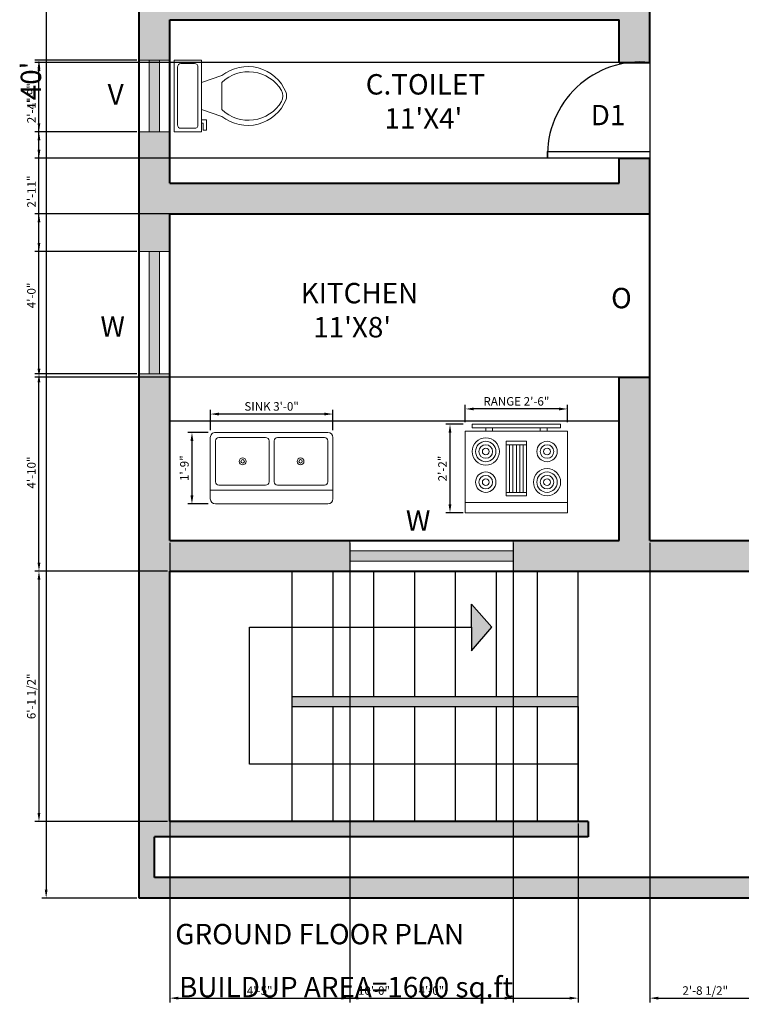
# Model space of a CAD drawing. Units: inches. Extents: x 4432 to 4859, y 8121 to 8698.
# Tile 1 of 4: x 4432 to 4644, y 8121 to 8410. Entities that reach past the tile are written whole.
import ezdxf

# ---------------------------------------------------------------- set-up
doc = ezdxf.new("R2010")
doc.units = ezdxf.units.IN
for name, color, linetype, lineweight in [('A-ANNO-DIMS', 2, 'Continuous', 18), ('A-ANNO-TEXT', 7, 'Continuous', 18), ('A-AREA-IDEN', 4, 'Continuous', 18), ('A-DOOR', 3, 'Continuous', 25), ('A-EQPM', 8, 'Continuous', 18), ('A-FLOR-CASE', 8, 'Continuous', 25), ('A-FLOR-FIXT', 9, 'Continuous', 18), ('A-FLOR-STRS', 7, 'Continuous', 25), ('A-FURN-PATT', 8, 'Continuous', 13), ('A-GLAZ', 4, 'Continuous', 20), ('A-GLAZ-PATT', 4, 'Continuous', 13), ('A-WALL', 7, 'Continuous', 40)]:
    doc.layers.add(name, color=color, linetype=linetype, lineweight=lineweight)
doc.layers.add('A-FLOR-PATT', color=219, linetype='Continuous', lineweight=13, true_color=0x642165)
doc.layers.add('A-WALL-PATT', color=219, linetype='Continuous', lineweight=13, true_color=0x642165)
doc.styles.get("Standard").update_dxf_attribs({"font": 'arial.ttf'})
doc.dimstyles.new('ISO-25', dxfattribs={"dimtxt": 2.5, "dimasz": 2.5, "dimexe": 1.25, "dimexo": 0.625, "dimtad": 1, "dimlunit": 3, "dimtxsty": 'Standard', "dimcen": 2.5, "dimadec": 0, "dimazin": 0, "dimtfac": 1, "dimtmove": 0, "dimatfit": 3, "dimfxl": 1, "dimarcsym": 0})

# ---------------------------------------------------------------- blocks, each defined once
blk = doc.blocks.new('Range-Oven - 30 in top')
for p, q in [((0, -3), (30, -3)), ((12, -6), (18, -6)), ((13, -20), (13, -6)), ((14, -6), (14, -20)), ((15, -20), (15, -6)), ((16, -6), (16, -20)), ((17, -20), (17, -6)), ((18, -20), (12, -20)), ((6, -24), (6, -25)), ((8, -25), (8, -24)), ((22, -25), (22, -24)), ((24, -24), (24, -25))]:
    blk.add_line(p, q)
for points in [[(0, -24), (0, 0), (30, 0), (30, -24)], [(12, -21), (12, -5), (18, -5), (18, -21)], [(2, -26), (2, -25), (28, -25), (28, -26)]]:
    blk.add_lwpolyline(points, close=True)
for centre, radius in [((6, -9), 4), ((6, -9), 3), ((6, -9), 2), ((6, -9), 1), ((24, -9), 3), ((24, -9), 2), ((24, -9), 1), ((24, -18), 4), ((6, -18), 3), ((6, -18), 2), ((6, -18), 1), ((24, -18), 3), ((24, -18), 2), ((24, -18), 1)]:
    blk.add_circle(centre, radius)
blk = doc.blocks.new('Sink-double - 36 in top')
for p, q in [((-18, -4), (18, -4)), ((-0.75, -18.5), (-0.75, -6.5)), ((0.75, -6.5), (0.75, -18.5))]:
    blk.add_line(p, q)
for points in [[(-16.5, 0), (16.5, 0)], [(-18, -19.5), (-18, -1.5)], [(18, -1.5), (18, -19.5)], [(-15.5, -5.5), (-1.75, -5.5)], [(1.75, -5.5), (15.5, -5.5)], [(-16.5, -18.5), (-16.5, -6.5)], [(16.5, -6.5), (16.5, -18.5)], [(-1.75, -19.5), (-15.5, -19.5)], [(15.5, -19.5), (1.75, -19.5)], [(16.5, -21), (-16.5, -21)]]:
    blk.add_lwpolyline(points)
for centre, radius in [((-8.5, -12.5), 1), ((8.5, -12.5), 1), ((-8.5, -12.5), 0.5), ((8.5, -12.5), 0.5)]:
    blk.add_circle(centre, radius)
for centre, radius, start, end in [((-16.5, -1.5), 1.5, 90, 180), ((16.5, -1.5), 1.5, 0, 90), ((-15.5, -6.5), 1, 90, 180), ((-1.75, -6.5), 1, 0, 90), ((1.75, -6.5), 1, 90, 180), ((15.5, -6.5), 1, 0, 90), ((-16.5, -19.5), 1.5, 180, 270), ((-15.5, -18.5), 1, 180, 270), ((-1.75, -18.5), 1, 270, 0), ((1.75, -18.5), 1, 180, 270), ((15.5, -18.5), 1, 270, 0), ((16.5, -19.5), 1.5, 270, 0)]:
    blk.add_arc(centre, radius, start, end)
blk = doc.blocks.new('Toilet - top')
for p, q in [((9.5, -6), (9.5, -2)), ((-10, -8.5), (-8, -8.5)), ((-10, -9.5), (-10, -8.5)), ((-8, -8.5), (-8, -8)), ((-7, -8), (-7, -9.5)), ((-4, -8), (-6, -14)), ((4, -8), (6, -14)), ((-7, -9.5), (-10, -9.5)), ((4, -14), (-4, -14))]:
    blk.add_line(p, q)
blk.add_lwpolyline([(10.5, -8), (10.5, 0), (-10.5, 0), (-10.5, -8)], close=True)
for points in [[(-9.5, -2), (-9.5, -6)], [(8.5, -1), (-8.5, -1)], [(-8.5, -7), (8.5, -7)]]:
    blk.add_lwpolyline(points)
for centre, radius, start, end in [((-8.62, -1.88), 0.884, 81.8699, 188.1301), ((8.62, -1.88), 0.884, 351.8699, 98.1301), ((-8.62, -6.12), 0.884, 171.8699, 278.1301), ((8.62, -6.12), 0.884, 261.8699, 8.1301), ((3.52, -21.58), 12.17, 141.4691, 247.9714), ((4.2, -21.82), 11.33, 136.3677, 238.9468), ((-3.52, -21.58), 12.17, 292.0284, 38.5307), ((-4.2, -21.82), 11.33, 301.053, 43.6321), ((0, -27.88), 4, 245.7318, 294.2682), ((0, -29), 4, 254.8605, 285.1395)]:
    blk.add_arc(centre, radius, start, end)
blk = doc.blocks.new('*D15')
at = {"layer": 'A-ANNO-DIMS', "color": 0, "lineweight": -2, "transparency": 16777216}
for p, q in [((4466.84, 8631.96), (4438.93, 8631.96)), ((4440.18, 8629.46), (4440.18, 8154.46)), ((4466.84, 8151.96), (4438.93, 8151.96))]:
    blk.add_line(p, q, dxfattribs=at)
at = {"layer": 'A-ANNO-DIMS', "color": 0, "transparency": 16777216}
for points in [[(4439.77, 8629.46), (4440.6, 8629.46), (4440.18, 8631.96)], [(4439.77, 8154.46), (4440.6, 8154.46), (4440.18, 8151.96)]]:
    blk.add_solid(points, dxfattribs=at)
at = {"layer": 'Defpoints', "color": 0, "transparency": 16777216}
for p in [(4467.47, 8631.96), (4440.18, 8151.96), (4467.47, 8151.96)]:
    blk.add_point(p, dxfattribs=at)
at = {"layer": 'A-ANNO-DIMS', "color": 0, "transparency": 16777216, "insert": (4436.49, 8391.96), "char_height": 6, "attachment_point": 5, "rotation": 90}
blk.add_mtext("40'", dxfattribs=at)
blk = doc.blocks.new('WIN-36IN')
for p, q in [((0, 0), (0, 9)), ((0, 9), (36, 9)), ((36, 9), (36, 0)), ((0, 6), (36, 6)), ((0, 3), (36, 3)), ((36, 0), (0, 0))]:
    blk.add_line(p, q)
blk = doc.blocks.new('*D45')
at = {"layer": 'A-ANNO-DIMS', "color": 0, "lineweight": -2, "transparency": 16777216}
for p, q in [((4563.31, 8291.74), (4563.31, 8296.87)), ((4590.81, 8295.62), (4565.81, 8295.62)), ((4593.31, 8291.74), (4593.31, 8296.87))]:
    blk.add_line(p, q, dxfattribs=at)
at = {"layer": 'A-ANNO-DIMS', "color": 0, "transparency": 16777216}
for points in [[(4565.81, 8296.03), (4565.81, 8295.2), (4563.31, 8295.62)], [(4590.81, 8296.03), (4590.81, 8295.2), (4593.31, 8295.62)]]:
    blk.add_solid(points, dxfattribs=at)
at = {"layer": 'Defpoints', "color": 0, "transparency": 16777216}
for p in [(4563.31, 8295.62), (4563.31, 8291.12), (4593.31, 8291.12)]:
    blk.add_point(p, dxfattribs=at)
at = {"layer": 'A-ANNO-DIMS', "color": 0, "transparency": 16777216, "insert": (4578.31, 8297.53), "char_height": 2.5, "attachment_point": 5}
blk.add_mtext('RANGE 2\'-6"', dxfattribs=at)
blk = doc.blocks.new('*D46')
at = {"layer": 'A-ANNO-DIMS', "color": 0, "lineweight": -2, "transparency": 16777216}
for p, q in [((4562.69, 8291.12), (4557.56, 8291.12)), ((4558.81, 8288.62), (4558.81, 8267.62)), ((4562.69, 8265.12), (4557.56, 8265.12))]:
    blk.add_line(p, q, dxfattribs=at)
at = {"layer": 'A-ANNO-DIMS', "color": 0, "transparency": 16777216}
for points in [[(4558.39, 8288.62), (4559.23, 8288.62), (4558.81, 8291.12)], [(4558.39, 8267.62), (4559.23, 8267.62), (4558.81, 8265.12)]]:
    blk.add_solid(points, dxfattribs=at)
at = {"layer": 'Defpoints', "color": 0, "transparency": 16777216}
for p in [(4563.31, 8291.12), (4558.81, 8265.12), (4563.31, 8265.12)]:
    blk.add_point(p, dxfattribs=at)
at = {"layer": 'A-ANNO-DIMS', "color": 0, "transparency": 16777216, "insert": (4556.93, 8278.12), "char_height": 2.5, "attachment_point": 5, "rotation": 90}
blk.add_mtext('2\'-2"', dxfattribs=at)
blk = doc.blocks.new('*D47')
at = {"layer": 'A-ANNO-DIMS', "color": 0, "lineweight": -2, "transparency": 16777216}
for p, q in [((4488.41, 8289.35), (4488.41, 8295.37)), ((4524.41, 8289.35), (4524.41, 8295.37)), ((4521.91, 8294.12), (4490.91, 8294.12))]:
    blk.add_line(p, q, dxfattribs=at)
at = {"layer": 'A-ANNO-DIMS', "color": 0, "transparency": 16777216}
for points in [[(4490.91, 8294.54), (4490.91, 8293.71), (4488.41, 8294.12)], [(4521.91, 8294.54), (4521.91, 8293.71), (4524.41, 8294.12)]]:
    blk.add_solid(points, dxfattribs=at)
at = {"layer": 'Defpoints', "color": 0, "transparency": 16777216}
for p in [(4488.41, 8294.12), (4488.41, 8288.72), (4524.41, 8288.72)]:
    blk.add_point(p, dxfattribs=at)
at = {"layer": 'A-ANNO-DIMS', "color": 0, "transparency": 16777216, "insert": (4506.41, 8296.04), "char_height": 2.5, "attachment_point": 5}
blk.add_mtext('SINK 3\'-0"', dxfattribs=at)
blk = doc.blocks.new('*D48')
at = {"layer": 'A-ANNO-DIMS', "color": 0, "lineweight": -2, "transparency": 16777216}
for p, q in [((4487.78, 8288.72), (4481.76, 8288.72)), ((4483.01, 8286.22), (4483.01, 8270.22)), ((4487.78, 8267.72), (4481.76, 8267.72))]:
    blk.add_line(p, q, dxfattribs=at)
at = {"layer": 'A-ANNO-DIMS', "color": 0, "transparency": 16777216}
for points in [[(4482.59, 8286.22), (4483.42, 8286.22), (4483.01, 8288.72)], [(4482.59, 8270.22), (4483.42, 8270.22), (4483.01, 8267.72)]]:
    blk.add_solid(points, dxfattribs=at)
at = {"layer": 'Defpoints', "color": 0, "transparency": 16777216}
for p in [(4488.41, 8288.72), (4483.01, 8267.72), (4488.41, 8267.72)]:
    blk.add_point(p, dxfattribs=at)
at = {"layer": 'A-ANNO-DIMS', "color": 0, "transparency": 16777216, "insert": (4481.11, 8278.22), "char_height": 2.5, "attachment_point": 5, "rotation": 90}
blk.add_mtext('1\'-9"', dxfattribs=at)
blk = doc.blocks.new('*D58')
at = {"layer": 'A-ANNO-DIMS', "color": 0, "lineweight": -2, "transparency": 16777216}
for p, q in [((4476.47, 8173.83), (4476.47, 8121.31)), ((4596.47, 8173.83), (4596.47, 8121.31)), ((4478.97, 8122.56), (4593.97, 8122.56))]:
    blk.add_line(p, q, dxfattribs=at)
at = {"layer": 'A-ANNO-DIMS', "color": 0, "transparency": 16777216}
for points in [[(4478.97, 8122.97), (4478.97, 8122.14), (4476.47, 8122.56)], [(4593.97, 8122.97), (4593.97, 8122.14), (4596.47, 8122.56)]]:
    blk.add_solid(points, dxfattribs=at)
at = {"layer": 'Defpoints', "color": 0, "transparency": 16777216}
for p in [(4476.47, 8174.46), (4596.47, 8174.46), (4596.47, 8122.56)]:
    blk.add_point(p, dxfattribs=at)
at = {"layer": 'A-ANNO-DIMS', "color": 0, "transparency": 16777216, "insert": (4536.47, 8124.46), "char_height": 2.5, "attachment_point": 5}
blk.add_mtext('10\'-0"', dxfattribs=at)
blk = doc.blocks.new('*D59')
at = {"layer": 'A-ANNO-DIMS', "color": 0, "lineweight": -2, "transparency": 16777216}
for p, q in [((4475.84, 8247.96), (4436.82, 8247.96)), ((4438.07, 8245.46), (4438.07, 8176.96)), ((4475.84, 8174.46), (4436.82, 8174.46))]:
    blk.add_line(p, q, dxfattribs=at)
at = {"layer": 'A-ANNO-DIMS', "color": 0, "transparency": 16777216}
for points in [[(4437.65, 8245.46), (4438.48, 8245.46), (4438.07, 8247.96)], [(4437.65, 8176.96), (4438.48, 8176.96), (4438.07, 8174.46)]]:
    blk.add_solid(points, dxfattribs=at)
at = {"layer": 'Defpoints', "color": 0, "transparency": 16777216}
for p in [(4476.47, 8247.96), (4438.07, 8174.46), (4476.47, 8174.46)]:
    blk.add_point(p, dxfattribs=at)
at = {"layer": 'A-ANNO-DIMS', "color": 0, "transparency": 16777216, "insert": (4436.15, 8211.21), "char_height": 2.5, "attachment_point": 5, "rotation": 90}
blk.add_mtext('6\'-1 1/2"', dxfattribs=at)
blk = doc.blocks.new('*D60')
at = {"layer": 'A-ANNO-DIMS', "color": 0, "lineweight": -2, "transparency": 16777216}
for p, q in [((4476.47, 8256.33), (4476.47, 8121.31)), ((4529.35, 8256.33), (4529.35, 8121.31)), ((4478.97, 8122.56), (4526.85, 8122.56))]:
    blk.add_line(p, q, dxfattribs=at)
at = {"layer": 'A-ANNO-DIMS', "color": 0, "transparency": 16777216}
for points in [[(4478.97, 8122.97), (4478.97, 8122.14), (4476.47, 8122.56)], [(4526.85, 8122.97), (4526.85, 8122.14), (4529.35, 8122.56)]]:
    blk.add_solid(points, dxfattribs=at)
at = {"layer": 'Defpoints', "color": 0, "transparency": 16777216}
for p in [(4476.47, 8256.96), (4529.35, 8256.96), (4529.35, 8122.56)]:
    blk.add_point(p, dxfattribs=at)
at = {"layer": 'A-ANNO-DIMS', "color": 0, "transparency": 16777216, "insert": (4502.91, 8124.45), "char_height": 2.5, "attachment_point": 5}
blk.add_mtext('4\'-5"', dxfattribs=at)
blk = doc.blocks.new('*D61')
at = {"layer": 'A-ANNO-DIMS', "color": 0, "lineweight": -2, "transparency": 16777216}
for p, q in [((4529.35, 8256.33), (4529.35, 8121.31)), ((4577.35, 8256.33), (4577.35, 8121.31)), ((4531.85, 8122.56), (4574.85, 8122.56))]:
    blk.add_line(p, q, dxfattribs=at)
at = {"layer": 'A-ANNO-DIMS', "color": 0, "transparency": 16777216}
for points in [[(4531.85, 8122.97), (4531.85, 8122.14), (4529.35, 8122.56)], [(4574.85, 8122.97), (4574.85, 8122.14), (4577.35, 8122.56)]]:
    blk.add_solid(points, dxfattribs=at)
at = {"layer": 'Defpoints', "color": 0, "transparency": 16777216}
for p in [(4529.35, 8256.96), (4577.35, 8256.96), (4577.35, 8122.56)]:
    blk.add_point(p, dxfattribs=at)
at = {"layer": 'A-ANNO-DIMS', "color": 0, "transparency": 16777216, "insert": (4553.35, 8124.46), "char_height": 2.5, "attachment_point": 5}
blk.add_mtext('4\'-0"', dxfattribs=at)
blk = doc.blocks.new('*D62')
at = {"layer": 'A-ANNO-DIMS', "color": 0, "lineweight": -2, "transparency": 16777216}
for p, q in [((4617.47, 8256.33), (4617.47, 8121.31)), ((4650.1, 8247.33), (4650.1, 8121.31)), ((4619.97, 8122.56), (4647.6, 8122.56))]:
    blk.add_line(p, q, dxfattribs=at)
at = {"layer": 'A-ANNO-DIMS', "color": 0, "transparency": 16777216}
for points in [[(4619.97, 8122.97), (4619.97, 8122.14), (4617.47, 8122.56)], [(4647.6, 8122.97), (4647.6, 8122.14), (4650.1, 8122.56)]]:
    blk.add_solid(points, dxfattribs=at)
at = {"layer": 'Defpoints', "color": 0, "transparency": 16777216}
for p in [(4617.47, 8256.96), (4650.1, 8247.96), (4650.1, 8122.56)]:
    blk.add_point(p, dxfattribs=at)
at = {"layer": 'A-ANNO-DIMS', "color": 0, "transparency": 16777216, "insert": (4633.79, 8124.47), "char_height": 2.5, "attachment_point": 5}
blk.add_mtext('2\'-8 1/2"', dxfattribs=at)
blk = doc.blocks.new('*D66')
at = {"layer": 'A-ANNO-DIMS', "color": 0, "lineweight": -2, "transparency": 16777216}
for p, q in [((4466.84, 8305.9), (4436.82, 8305.9)), ((4438.07, 8250.46), (4438.07, 8303.4)), ((4475.84, 8247.96), (4436.82, 8247.96))]:
    blk.add_line(p, q, dxfattribs=at)
at = {"layer": 'A-ANNO-DIMS', "color": 0, "transparency": 16777216}
for points in [[(4437.65, 8303.4), (4438.48, 8303.4), (4438.07, 8305.9)], [(4437.65, 8250.46), (4438.48, 8250.46), (4438.07, 8247.96)]]:
    blk.add_solid(points, dxfattribs=at)
at = {"layer": 'Defpoints', "color": 0, "transparency": 16777216}
for p in [(4438.07, 8305.9), (4467.47, 8305.9), (4476.47, 8247.96)]:
    blk.add_point(p, dxfattribs=at)
at = {"layer": 'A-ANNO-DIMS', "color": 0, "transparency": 16777216, "insert": (4436.17, 8276.93), "char_height": 2.5, "attachment_point": 5, "rotation": 90}
blk.add_mtext('4\'-10"', dxfattribs=at)
blk = doc.blocks.new('*D67')
at = {"layer": 'A-ANNO-DIMS', "color": 0, "lineweight": -2, "transparency": 16777216}
for p, q in [((4466.84, 8377.05), (4436.82, 8377.05)), ((4438.07, 8344.4), (4438.07, 8374.55)), ((4466.84, 8341.9), (4436.82, 8341.9))]:
    blk.add_line(p, q, dxfattribs=at)
at = {"layer": 'A-ANNO-DIMS', "color": 0, "transparency": 16777216}
for points in [[(4437.65, 8374.55), (4438.48, 8374.55), (4438.07, 8377.05)], [(4437.65, 8344.4), (4438.48, 8344.4), (4438.07, 8341.9)]]:
    blk.add_solid(points, dxfattribs=at)
at = {"layer": 'Defpoints', "color": 0, "transparency": 16777216}
for p in [(4438.07, 8377.05), (4467.47, 8377.05), (4467.47, 8341.9)]:
    blk.add_point(p, dxfattribs=at)
at = {"layer": 'A-ANNO-DIMS', "color": 0, "transparency": 16777216, "insert": (4436.19, 8359.47), "char_height": 2.5, "attachment_point": 5, "rotation": 90}
blk.add_mtext('2\'-11"', dxfattribs=at)
blk = doc.blocks.new('*D68')
at = {"layer": 'A-ANNO-DIMS', "color": 0, "lineweight": -2, "transparency": 16777216}
for p, q in [((4466.84, 8398.05), (4436.82, 8398.05)), ((4438.07, 8379.55), (4438.07, 8395.55)), ((4466.84, 8377.05), (4436.82, 8377.05))]:
    blk.add_line(p, q, dxfattribs=at)
at = {"layer": 'A-ANNO-DIMS', "color": 0, "transparency": 16777216}
for points in [[(4437.65, 8395.55), (4438.48, 8395.55), (4438.07, 8398.05)], [(4437.65, 8379.55), (4438.48, 8379.55), (4438.07, 8377.05)]]:
    blk.add_solid(points, dxfattribs=at)
at = {"layer": 'Defpoints', "color": 0, "transparency": 16777216}
for p in [(4438.07, 8398.05), (4467.47, 8398.05), (4467.47, 8377.05)]:
    blk.add_point(p, dxfattribs=at)
at = {"layer": 'A-ANNO-DIMS', "color": 0, "transparency": 16777216, "insert": (4436.17, 8387.55), "char_height": 2.5, "attachment_point": 5, "rotation": 90}
blk.add_mtext('1\'-9"', dxfattribs=at)
blk = doc.blocks.new('*D70')
at = {"layer": 'A-ANNO-DIMS', "color": 0, "lineweight": -2, "transparency": 16777216}
for p, q in [((4616.84, 8352.96), (4436.82, 8352.96)), ((4438.07, 8307.46), (4438.07, 8350.46)), ((4616.84, 8304.96), (4436.82, 8304.96))]:
    blk.add_line(p, q, dxfattribs=at)
at = {"layer": 'A-ANNO-DIMS', "color": 0, "transparency": 16777216}
for points in [[(4437.65, 8350.46), (4438.48, 8350.46), (4438.07, 8352.96)], [(4437.65, 8307.46), (4438.48, 8307.46), (4438.07, 8304.96)]]:
    blk.add_solid(points, dxfattribs=at)
at = {"layer": 'Defpoints', "color": 0, "transparency": 16777216}
for p in [(4438.07, 8352.96), (4617.47, 8352.96), (4617.47, 8304.96)]:
    blk.add_point(p, dxfattribs=at)
at = {"layer": 'A-ANNO-DIMS', "color": 0, "transparency": 16777216, "insert": (4436.17, 8328.96), "char_height": 2.5, "attachment_point": 5, "rotation": 90}
blk.add_mtext('4\'-0"', dxfattribs=at)
blk = doc.blocks.new('*D72')
at = {"layer": 'A-ANNO-DIMS', "color": 0, "lineweight": -2, "transparency": 16777216}
for p, q in [((4616.84, 8397.41), (4436.82, 8397.41)), ((4438.07, 8371.74), (4438.07, 8394.91)), ((4616.84, 8369.24), (4436.82, 8369.24))]:
    blk.add_line(p, q, dxfattribs=at)
at = {"layer": 'A-ANNO-DIMS', "color": 0, "transparency": 16777216}
for points in [[(4437.65, 8394.91), (4438.48, 8394.91), (4438.07, 8397.41)], [(4437.65, 8371.74), (4438.48, 8371.74), (4438.07, 8369.24)]]:
    blk.add_solid(points, dxfattribs=at)
at = {"layer": 'Defpoints', "color": 0, "transparency": 16777216}
for p in [(4438.07, 8397.41), (4617.47, 8397.41), (4617.47, 8369.24)]:
    blk.add_point(p, dxfattribs=at)
at = {"layer": 'A-ANNO-DIMS', "color": 0, "transparency": 16777216, "insert": (4436.19, 8383.32), "char_height": 2.5, "attachment_point": 5, "rotation": 90}
blk.add_mtext('2\'-4"', dxfattribs=at)

msp = doc.modelspace()

# ---------------------------------------------------------------- hatches: boundary and pattern name
at = {"layer": 'A-FLOR-PATT'}
h = msp.add_hatch(color=256, dxfattribs=at)
h.dxf.hatch_style = 1
h.paths.add_polyline_path([(4596.468, 8211.206), (4512.468, 8211.206), (4512.468, 8208.206), (4596.468, 8208.206)])
h.paths.add_polyline_path([(4571.133, 8231.507), (4565.158, 8238.304), (4565.158, 8231.507), (4565.158, 8224.58)])
at = {"layer": 'A-FURN-PATT'}
h = msp.add_hatch(dxfattribs=at)
h.set_pattern_fill('CROSS', color=256)
h.paths.add_polyline_path([(4558.735, 8563.044), (4508.335, 8563.044), (4508.335, 8547.844), (4495.535, 8547.844), (4495.535, 8503.044), (4558.735, 8503.044)])
h.paths.add_polyline_path([(4768.654, 8563.044), (4718.254, 8563.044), (4718.254, 8547.844), (4705.454, 8547.844), (4705.454, 8503.044), (4768.654, 8503.044)])
h.paths.add_polyline_path([(4699.088, 8354.439, 1), (4726.919, 8354.439, 1)])
at = {"layer": 'A-GLAZ-PATT'}
h = msp.add_hatch(color=256, dxfattribs=at)
h.dxf.hatch_style = 1
h.paths.add_polyline_path([(4592.313, 8628.956), (4556.313, 8628.956), (4556.313, 8625.956), (4592.313, 8625.956)])
h.paths.add_polyline_path([(4660.176, 8628.956), (4636.176, 8628.956), (4636.176, 8625.956), (4660.176, 8625.956)])
h.paths.add_polyline_path([(4799.877, 8628.956), (4763.877, 8628.956), (4763.877, 8625.956), (4799.877, 8625.956)])
h.paths.add_polyline_path([(4473.468, 8508.361), (4470.468, 8508.361), (4470.468, 8448.361), (4473.468, 8448.361)])
h.paths.add_polyline_path([(4473.468, 8398.047), (4470.468, 8398.047), (4470.468, 8377.047), (4473.468, 8377.047)])
h.paths.add_polyline_path([(4473.468, 8341.903), (4470.468, 8341.903), (4470.468, 8305.903), (4473.468, 8305.903)])
h.paths.add_polyline_path([(4577.354, 8253.956), (4529.354, 8253.956), (4529.354, 8250.956), (4577.354, 8250.956)])
h.paths.add_polyline_path([(4662.104, 8253.956), (4650.104, 8253.956), (4650.104, 8250.956), (4662.104, 8250.956)])
h.paths.add_polyline_path([(4722.104, 8253.956), (4710.104, 8253.956), (4710.104, 8250.956), (4722.104, 8250.956)])
h.paths.add_polyline_path([(4824.468, 8397.007), (4821.468, 8397.007), (4821.468, 8361.007), (4824.468, 8361.007)])
h.paths.add_polyline_path([(4824.468, 8509.871), (4821.468, 8509.871), (4821.468, 8449.871), (4824.468, 8449.871)])
at = {"layer": 'A-WALL-PATT'}
h = msp.add_hatch(color=256, dxfattribs=at)
h.dxf.hatch_style = 1
h.paths.add_polyline_path([(4556.313, 8631.956), (4467.468, 8631.956), (4467.468, 8508.361), (4476.468, 8508.361), (4476.468, 8622.956), (4556.313, 8622.956)])
h.paths.add_polyline_path([(4636.176, 8631.956), (4592.313, 8631.956), (4592.313, 8622.956), (4608.468, 8622.956), (4608.468, 8546.941), (4617.468, 8546.941), (4617.468, 8622.956), (4636.176, 8622.956)])
h.paths.add_polyline_path([(4763.877, 8631.956), (4660.176, 8631.956), (4660.176, 8622.956), (4677.468, 8622.956), (4677.468, 8502.956), (4617.468, 8502.956), (4617.468, 8524.355), (4608.468, 8524.355), (4608.468, 8459.776), (4615.468, 8459.776, -0.0172363), (4617.468, 8459.776), (4617.468, 8493.956), (4677.468, 8493.956), (4677.468, 8459.776, -0.0172363), (4679.468, 8459.776), (4686.468, 8459.776), (4686.468, 8622.956), (4763.877, 8622.956)])
h.paths.add_polyline_path([(4827.468, 8631.956), (4799.877, 8631.956), (4799.877, 8622.956), (4818.468, 8622.956), (4818.468, 8509.871), (4827.468, 8509.871)])
h.paths.add_polyline_path([(4617.468, 8429.776), (4608.468, 8429.776), (4608.468, 8418.956), (4476.468, 8418.956), (4476.468, 8448.361), (4467.468, 8448.361), (4467.468, 8398.047), (4476.468, 8398.047), (4476.468, 8409.956), (4608.468, 8409.956), (4608.468, 8397.41), (4612.05, 8397.41, -0.0497121), (4617.468, 8397.41)])
h.paths.add_polyline_path([(4827.468, 8449.871), (4818.468, 8449.871), (4818.468, 8418.956), (4686.468, 8418.956), (4686.468, 8429.776), (4677.468, 8429.776), (4677.468, 8409.956), (4818.468, 8409.956), (4818.468, 8397.007), (4827.468, 8397.007)])
h.paths.add_polyline_path([(4617.468, 8369.235), (4608.468, 8369.235), (4608.468, 8361.956), (4476.468, 8361.956), (4476.468, 8377.047), (4467.468, 8377.047), (4467.468, 8341.903), (4476.468, 8341.903), (4476.468, 8352.956), (4617.468, 8352.956)])
h.paths.add_polyline_path([(4529.354, 8256.956), (4476.468, 8256.956), (4476.468, 8305.903), (4467.468, 8305.903), (4467.468, 8151.956), (4650.104, 8151.956), (4650.104, 8157.956), (4471.968, 8157.956), (4471.968, 8169.956), (4599.396, 8169.956), (4599.396, 8174.456), (4476.468, 8174.456), (4476.468, 8247.956), (4529.354, 8247.956)])
h.paths.add_polyline_path([(4650.104, 8256.956), (4617.468, 8256.956), (4617.468, 8304.956), (4608.468, 8304.956), (4608.468, 8256.956), (4577.354, 8256.956), (4577.354, 8247.956), (4650.104, 8247.956)], flags=17)
h.paths.add_polyline_path([(4827.468, 8361.007), (4818.468, 8361.007), (4818.468, 8333.456), (4807.435, 8333.456, -0.0172363), (4807.435, 8331.456), (4807.435, 8328.956), (4818.468, 8328.956), (4818.468, 8256.956), (4770.468, 8256.956), (4770.468, 8328.956), (4777.435, 8328.956), (4777.435, 8333.456), (4765.968, 8333.456), (4765.968, 8256.956), (4722.104, 8256.956), (4722.104, 8247.956), (4821.468, 8247.956), (4821.468, 8157.956), (4765.968, 8157.956), (4765.968, 8151.956), (4827.468, 8151.956)])
h.paths.add_polyline_path([(4765.968, 8154.956), (4650.104, 8154.956), (4650.104, 8151.956), (4765.968, 8151.956)])

# ---------------------------------------------------------------- linework, layer by layer
at = {"layer": 'A-DOOR'}
for p, q in [((4617.468, 8397.41), (4617.468, 8369.235)), ((4587.468, 8369.235), (4587.468, 8371.235)), ((4587.468, 8371.235), (4617.468, 8371.235)), ((4617.468, 8369.235), (4587.468, 8369.235))]:
    msp.add_line(p, q, dxfattribs=at)
msp.add_arc((4614.759, 8370.235), 27.31, 84.30809, 182.09847, dxfattribs=at)
at = {"layer": 'A-FLOR-CASE'}
msp.add_line((4608.468, 8291.999), (4476.468, 8291.999), dxfattribs=at)
at = {"layer": 'A-FLOR-STRS'}
for p, q in [((4512.468, 8174.456), (4512.468, 8247.956)), ((4524.468, 8211.206), (4524.468, 8247.956)), ((4536.468, 8211.206), (4536.468, 8247.956)), ((4536.468, 8211.206), (4536.468, 8247.956)), ((4548.468, 8211.206), (4548.468, 8247.956)), ((4560.468, 8211.206), (4560.468, 8247.956)), ((4572.468, 8211.206), (4572.468, 8247.956)), ((4584.468, 8211.206), (4584.468, 8247.956)), ((4596.468, 8174.456), (4596.468, 8247.956)), ((4565.158, 8231.507), (4565.158, 8238.304)), ((4571.133, 8231.507), (4565.158, 8238.304)), ((4499.867, 8191.331), (4499.867, 8231.507)), ((4499.867, 8231.507), (4565.158, 8231.507)), ((4565.158, 8231.507), (4565.158, 8224.58)), ((4565.158, 8224.58), (4571.133, 8231.507)), ((4512.468, 8211.206), (4596.468, 8211.206)), ((4512.468, 8208.206), (4596.468, 8208.206)), ((4524.468, 8174.456), (4524.468, 8208.206)), ((4536.468, 8174.456), (4536.468, 8208.206)), ((4536.468, 8174.456), (4536.468, 8208.206)), ((4548.468, 8174.456), (4548.468, 8208.206)), ((4560.468, 8174.456), (4560.468, 8208.206)), ((4572.468, 8174.456), (4572.468, 8208.206)), ((4584.468, 8174.456), (4584.468, 8208.206)), ((4596.468, 8208.206), (4596.468, 8174.456)), ((4596.468, 8191.331), (4499.867, 8191.331)), ((4596.468, 8174.456), (4596.468, 8191.331))]:
    msp.add_line(p, q, dxfattribs=at)
at = {"layer": 'A-GLAZ'}
for p, q in [((4467.468, 8377.047), (4467.468, 8398.047)), ((4467.468, 8398.047), (4476.468, 8398.047)), ((4467.468, 8377.047), (4467.468, 8398.047)), ((4470.468, 8377.047), (4470.468, 8398.047)), ((4473.468, 8377.047), (4473.468, 8398.047)), ((4476.468, 8377.047), (4476.468, 8398.047)), ((4476.468, 8377.047), (4467.468, 8377.047)), ((4467.468, 8305.903), (4476.468, 8305.903)), ((4529.354, 8256.956), (4529.354, 8247.956)), ((4529.354, 8256.956), (4577.354, 8256.956)), ((4577.354, 8256.956), (4577.354, 8247.956)), ((4529.354, 8253.956), (4577.354, 8253.956)), ((4529.354, 8250.956), (4577.354, 8250.956)), ((4529.354, 8247.956), (4577.354, 8247.956))]:
    msp.add_line(p, q, dxfattribs=at)
at = {"layer": 'A-WALL'}
for p, q in [((4467.468, 8151.956), (4467.468, 8631.956)), ((4617.468, 8397.41), (4617.468, 8429.776)), ((4476.468, 8409.956), (4608.468, 8409.956)), ((4476.468, 8361.956), (4476.468, 8409.956)), ((4608.468, 8397.41), (4608.468, 8409.956)), ((4608.468, 8397.41), (4617.468, 8397.41)), ((4608.468, 8369.235), (4617.468, 8369.235)), ((4608.468, 8361.956), (4608.468, 8369.235)), ((4617.468, 8256.956), (4617.468, 8369.235)), ((4476.468, 8361.956), (4608.468, 8361.956)), ((4476.468, 8352.956), (4617.468, 8352.956)), ((4476.468, 8256.956), (4476.468, 8352.956)), ((4608.468, 8256.956), (4608.468, 8304.956)), ((4608.468, 8304.956), (4617.468, 8304.956)), ((4476.468, 8256.956), (4608.468, 8256.956)), ((4476.468, 8256.956), (4608.468, 8256.956)), ((4617.468, 8256.956), (4662.104, 8256.956)), ((4476.468, 8247.956), (4821.468, 8247.956)), ((4476.468, 8174.456), (4476.468, 8247.956)), ((4599.396, 8174.456), (4476.468, 8174.456)), ((4599.396, 8174.456), (4599.396, 8169.956)), ((4599.396, 8169.956), (4471.968, 8169.956)), ((4471.968, 8157.956), (4471.968, 8169.956)), ((4650.104, 8157.956), (4471.968, 8157.956)), ((4827.468, 8151.956), (4467.468, 8151.956))]:
    msp.add_line(p, q, dxfattribs=at)

# ---------------------------------------------------------------- block references
at = {"layer": 'A-EQPM', "rotation": 180}
msp.add_blockref('Range-Oven - 30 in top', (4593.311, 8265.115), dxfattribs=at)
at = {"layer": 'A-FLOR-FIXT'}
for name, p, rotation in [('Toilet - top', (4477.781, 8387.547), 90), ('Sink-double - 36 in top', (4506.407, 8267.724), 180)]:
    msp.add_blockref(name, p, dxfattribs=dict(at, rotation=rotation))
at = {"layer": 'A-GLAZ', "rotation": 89.99999999999046}
msp.add_blockref('WIN-36IN', (4476.468, 8305.903), dxfattribs=at)

# ---------------------------------------------------------------- texts
at = {"layer": 'A-ANNO-TEXT', "char_height": 6, "attachment_point": 1}
for s, insert in [('V', (4458.238, 8391.024)), ('D1', (4600.148, 8384.946)), ('O', (4606.133, 8331.186)), ('W  ', (4456.12, 8322.849)), ('W  ', (4545.86, 8265.82)), (' GROUND FLOOR PLAN', (4476.278, 8144.37)), ('BUILDUP AREA=1600 sq.ft', (4479.216, 8128.795))]:
    msp.add_mtext_dynamic_manual_height_columns(s, width=117.51606, gutter_width=12.5, heights=[0], dxfattribs=dict(at, insert=insert))
at = {"layer": 'A-AREA-IDEN', "char_height": 6, "attachment_point": 1}
for s, insert in [(" {C.TOILET\\P    11'X4'}", (4532.228, 8393.97)), (" {KITCHEN\\P   11'X8'}", (4513.131, 8332.639))]:
    msp.add_mtext_dynamic_manual_height_columns(s, width=117.51606, gutter_width=12.5, heights=[0], dxfattribs=dict(at, insert=insert))

# ---------------------------------------------------------------- dimensions: what is measured, and where the dimension line sits
at = {"layer": 'A-ANNO-DIMS'}
for base, p1, p2, angle, override, picture, middle in [((4440.183, 8151.956), (4467.468, 8631.956), (4467.468, 8151.956), 90, {"dimtxt": 6, "dimclrd": 0, "dimclre": 0, "dimclrt": 0}, '*D15', (4436.494, 8391.956)), ((4438.068, 8398.047), (4467.468, 8377.047), (4467.468, 8398.047), 90, {"dimdec": 1, "dimlfac": 1, "dimrnd": 0, "dimzin": 1, "dimdsep": 46, "dimlunit": 4, "dimfrac": 2}, '*D68', (4436.166, 8387.547)), ((4438.068, 8397.41), (4617.468, 8369.235), (4617.468, 8397.41), 90, {"dimdec": 1, "dimlfac": 1, "dimrnd": 0, "dimzin": 1, "dimdsep": 46, "dimlunit": 4, "dimfrac": 2}, '*D72', (4436.187, 8383.323)), ((4438.068, 8377.047), (4467.468, 8341.903), (4467.468, 8377.047), 90, {"dimdec": 1, "dimlfac": 1, "dimrnd": 0, "dimzin": 1, "dimdsep": 46, "dimlunit": 4, "dimfrac": 2}, '*D67', (4436.187, 8359.475)), ((4438.068, 8352.956), (4617.468, 8304.956), (4617.468, 8352.956), 90, {"dimdec": 1, "dimlfac": 1, "dimrnd": 0, "dimzin": 1, "dimdsep": 46, "dimlunit": 4, "dimfrac": 2}, '*D70', (4436.166, 8328.956)), ((4438.068, 8305.903), (4476.468, 8247.956), (4467.468, 8305.903), 90, {"dimdec": 1, "dimlfac": 1, "dimrnd": 0, "dimzin": 1, "dimdsep": 46, "dimlunit": 4, "dimfrac": 2}, '*D66', (4436.166, 8276.93)), ((4558.811, 8265.115), (4563.311, 8291.115), (4563.311, 8265.115), 270, {"dimdec": 1, "dimlfac": 1, "dimrnd": 0, "dimzin": 1, "dimdsep": 46, "dimlunit": 4, "dimfrac": 2}, '*D46', (4556.931, 8278.115)), ((4483.007, 8267.724), (4488.407, 8288.724), (4488.407, 8267.724), 270, {"dimdec": 1, "dimlfac": 1, "dimrnd": 0, "dimzin": 1, "dimdsep": 46, "dimlunit": 4, "dimfrac": 2}, '*D48', (4481.105, 8278.224)), ((4438.068, 8174.456), (4476.468, 8247.956), (4476.468, 8174.456), 90, {"dimdec": 1, "dimlfac": 1, "dimrnd": 0, "dimzin": 1, "dimdsep": 46, "dimlunit": 4, "dimfrac": 2}, '*D59', (4436.15, 8211.206))]:
    dim = msp.add_linear_dim(base=base, p1=p1, p2=p2, angle=angle, dimstyle='ISO-25', override=override, dxfattribs=at)
    dim.commit()
    dim.dimension.update_dxf_attribs({"geometry": picture, "text_midpoint": middle})
for base, p1, p2, text, picture, middle in [((4563.311, 8295.615), (4593.311, 8291.115), (4563.311, 8291.115), 'RANGE <>', '*D45', (4578.311, 8297.533)), ((4488.407, 8294.124), (4524.407, 8288.724), (4488.407, 8288.724), 'SINK <>', '*D47', (4506.407, 8296.043))]:
    dim = msp.add_linear_dim(base=base, p1=p1, p2=p2, angle=180, text=text, dimstyle='ISO-25', override={"dimdec": 1, "dimlfac": 1, "dimrnd": 0, "dimzin": 1, "dimdsep": 46, "dimlunit": 4, "dimfrac": 2}, dxfattribs=at)
    dim.commit()
    dim.dimension.update_dxf_attribs({"geometry": picture, "text_midpoint": middle})
for base, p1, p2, picture, middle in [((4529.354, 8122.556), (4476.468, 8256.956), (4529.354, 8256.956), '*D60', (4502.911, 8124.453)), ((4577.354, 8122.556), (4529.354, 8256.956), (4577.354, 8256.956), '*D61', (4553.354, 8124.458)), ((4650.104, 8122.556), (4617.468, 8256.956), (4650.104, 8247.956), '*D62', (4633.786, 8124.474)), ((4596.468, 8122.556), (4476.468, 8174.456), (4596.468, 8174.456), '*D58', (4536.468, 8124.458))]:
    dim = msp.add_linear_dim(base=base, p1=p1, p2=p2, dimstyle='ISO-25', override={"dimdec": 1, "dimlfac": 1, "dimrnd": 0, "dimzin": 1, "dimdsep": 46, "dimlunit": 4, "dimfrac": 2}, dxfattribs=at)
    dim.commit()
    dim.dimension.update_dxf_attribs({"geometry": picture, "text_midpoint": middle})

doc.saveas('drawing.dxf')
